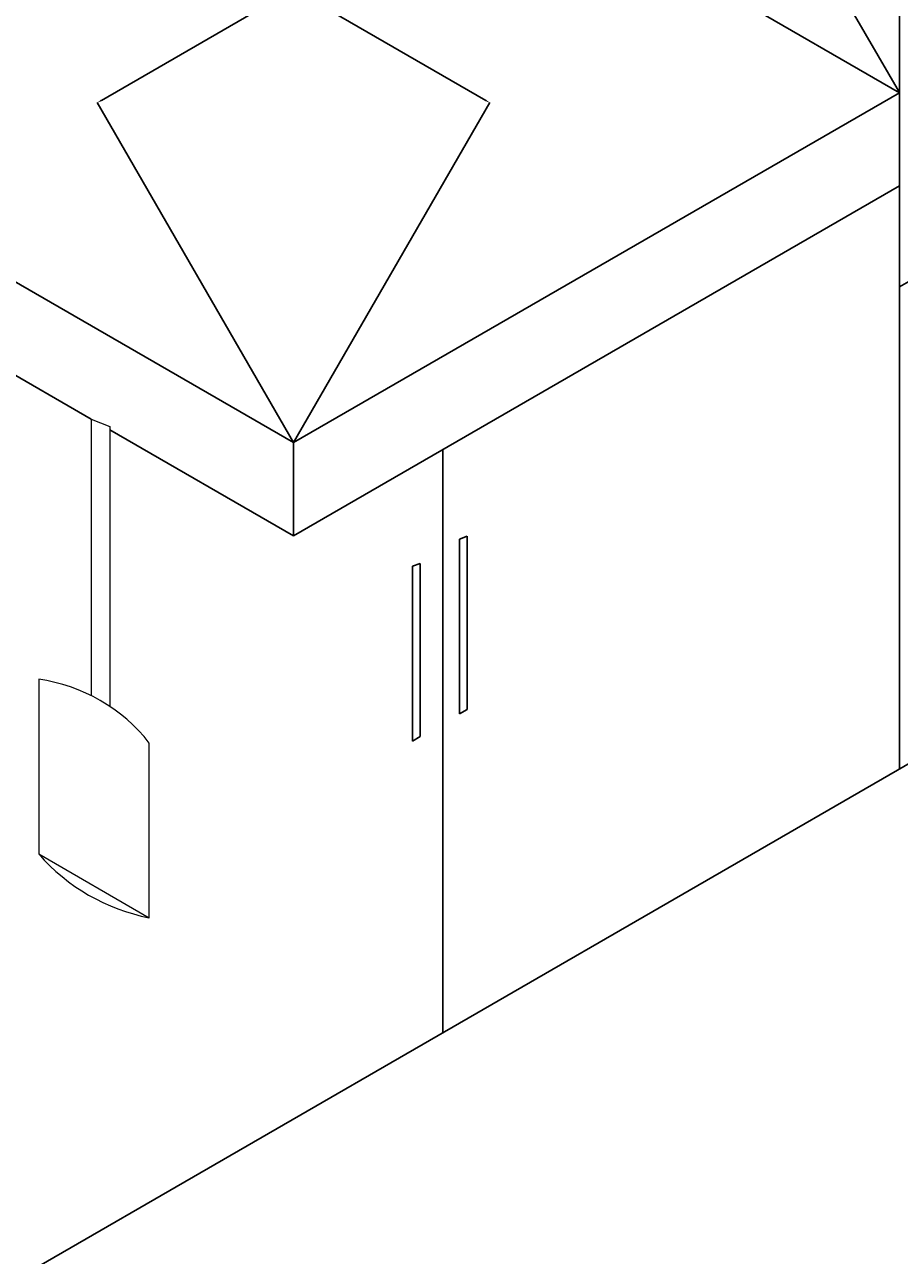
# Model space of a CAD drawing. Units: metres. Extents: x -2391 to 4922, y -635 to 4845.
# Tile 17 of 37: x -719 to 31, y 1408 to 2464. Entities that reach past the tile are written whole.
import ezdxf

# ---------------------------------------------------------------- set-up
doc = ezdxf.new("R2010")
doc.units = ezdxf.units.M
doc.header["$MEASUREMENT"] = 0
for name, color, linetype, lineweight in [('A-ANNO-DIMS', 2, 'Continuous', 18), ('A-EQPM', 9, 'Continuous', 18), ('A-FLOR-FIXT', 3, 'Continuous', 25)]:
    doc.layers.add(name, color=color, linetype=linetype, lineweight=lineweight)
doc.styles.get("Standard").update_dxf_attribs({"font": 'arial.ttf'})
doc.dimstyles.get("Standard").update_dxf_attribs({"dimtxt": 5, "dimasz": 4, "dimexe": 0.18, "dimexo": 0.0625, "dimgap": 0.09, "dimtad": 0, "dimtih": 1, "dimtoh": 1, "dimdec": 0, "dimzin": 0, "dimdsep": 46, "dimtxsty": 'Standard', "dimcen": 0.09, "dimadec": 0, "dimazin": 0, "dimtfac": 1, "dimtdec": 0, "dimtofl": 0, "dimtmove": 0, "dimatfit": 3, "dimfxl": 1, "dimtolj": 1, "dimtzin": 0, "dimarcsym": 0})

# ---------------------------------------------------------------- blocks, each defined once
blk = doc.blocks.new('UTENSIL-HANGING')
for p, q in [((0, 204.5), (0, 54.7)), ((94.7, 0), (94.7, 149.8)), ((0, 54.7), (94.7, 0))]:
    blk.add_line(p, q)
for centre, radius, start, end in [((-21.4, 58), 148.1, 38.3202, 81.6798), ((126.8, 165), 168.1, 221.0072, 258.9928)]:
    blk.add_arc(centre, radius, start, end)
blk = doc.blocks.new('HANDLE-DRAWER-152')
for p, q in [((6.8, 152.4), (0, 150)), ((0, 150), (0, 0)), ((6.8, 3.9), (6.8, 152.4)), ((0, 0), (6.8, 3.9))]:
    blk.add_line(p, q)
blk = doc.blocks.new('*D8')
at = {"layer": 'A-ANNO-DIMS', "color": 0, "lineweight": -2, "transparency": 16777216}
for p, q in [((-2047.3, 3005.2), (-2047.3, -631.4)), ((4577.8, 2350.2), (4577.8, -631.4)), ((-2043.3, -631.2), (1257.6, -631.2)), ((4573.8, -631.2), (1272.8, -631.2))]:
    blk.add_line(p, q, dxfattribs=at)
at = {"layer": 'A-ANNO-DIMS', "color": 0, "transparency": 16777216}
for points in [[(-2043.3, -630.6), (-2043.3, -631.9), (-2047.3, -631.2)], [(4573.8, -630.6), (4573.8, -631.9), (4577.8, -631.2)]]:
    blk.add_solid(points, dxfattribs=at)
at = {"layer": 'Defpoints', "color": 0, "transparency": 16777216}
for p in [(-2047.3, 3005.3), (4577.8, 2350.3), (4577.8, -631.2)]:
    blk.add_point(p, dxfattribs=at)
at = {"layer": 'A-ANNO-DIMS', "color": 0, "transparency": 16777216, "insert": (1265.2, -631.2), "char_height": 5, "attachment_point": 5}
blk.add_mtext('\\A1;6625', dxfattribs=at)
blk = doc.blocks.new('*D10')
at = {"layer": 'A-ANNO-DIMS', "color": 0, "lineweight": -2, "transparency": 16777216}
for p, q in [((550.7, 4505.3), (-2384, 4505.3)), ((-2383.8, 4501.3), (-2383.8, 2107.9)), ((-2383.8, -290.7), (-2383.8, 2102.6)), ((-488.6, -294.7), (-2384, -294.7))]:
    blk.add_line(p, q, dxfattribs=at)
at = {"layer": 'A-ANNO-DIMS', "color": 0, "transparency": 16777216}
for points in [[(-2384.5, 4501.3), (-2383.2, 4501.3), (-2383.8, 4505.3)], [(-2384.5, -290.7), (-2383.2, -290.7), (-2383.8, -294.7)]]:
    blk.add_solid(points, dxfattribs=at)
at = {"layer": 'Defpoints', "color": 0, "transparency": 16777216}
for p in [(-2383.8, 4505.3), (550.7, 4505.3), (-488.5, -294.7)]:
    blk.add_point(p, dxfattribs=at)
at = {"layer": 'A-ANNO-DIMS', "color": 0, "transparency": 16777216, "insert": (-2383.8, 2105.3), "char_height": 5, "attachment_point": 5}
blk.add_mtext('\\A1;4800', dxfattribs=at)
blk = doc.blocks.new('*D41')
at = {"layer": 'A-ANNO-DIMS', "color": 0, "lineweight": -2, "transparency": 16777216}
for p, q in [((-2047.3, 3005.3), (-1879, 3296.8)), ((-1875.6, 3294.7), (-1104.2, 2849.3)), ((-323.7, 2398.7), (-1095.1, 2844.1)), ((-488.5, 2105.3), (-320.1, 2396.8))]:
    blk.add_line(p, q, dxfattribs=at)
at = {"layer": 'A-ANNO-DIMS', "color": 0, "transparency": 16777216}
for points in [[(-1875.3, 3295.3), (-1876, 3294.1), (-1879.1, 3296.7)], [(-323.4, 2399.3), (-324, 2398.1), (-320.2, 2396.7)]]:
    blk.add_solid(points, dxfattribs=at)
at = {"layer": 'Defpoints', "color": 0, "transparency": 16777216}
for p in [(-2047.3, 3005.3), (-320.2, 2396.7), (-488.5, 2105.3)]:
    blk.add_point(p, dxfattribs=at)
at = {"layer": 'A-ANNO-DIMS', "color": 0, "transparency": 16777216, "insert": (-1099.7, 2846.7), "char_height": 5, "attachment_point": 5}
blk.add_mtext('\\A1;1800', dxfattribs=at)
blk = doc.blocks.new('*D42')
at = {"layer": 'A-ANNO-DIMS', "color": 0, "lineweight": -2, "transparency": 16777216}
for p, q in [((-140.6, 2694.7), (-392.4, 2549.3)), ((31.1, 2405.3), (-137.2, 2696.8)), ((-653.3, 2398.7), (-401.5, 2544.1)), ((-488.5, 2105.3), (-656.8, 2396.8))]:
    blk.add_line(p, q, dxfattribs=at)
at = {"layer": 'A-ANNO-DIMS', "color": 0, "transparency": 16777216}
for points in [[(-140.9, 2695.3), (-140.3, 2694.1), (-137.1, 2696.7)], [(-653.6, 2399.3), (-652.9, 2398.1), (-656.7, 2396.7)]]:
    blk.add_solid(points, dxfattribs=at)
at = {"layer": 'Defpoints', "color": 0, "transparency": 16777216}
for p in [(-137.1, 2696.7), (31.1, 2405.3), (-488.5, 2105.3)]:
    blk.add_point(p, dxfattribs=at)
at = {"layer": 'A-ANNO-DIMS', "color": 0, "transparency": 16777216, "insert": (-396.9, 2546.7), "char_height": 5, "attachment_point": 5}
blk.add_mtext('\\A1;600', dxfattribs=at)
blk = doc.blocks.new('*D46')
at = {"layer": 'A-ANNO-DIMS', "color": 0, "lineweight": -2, "transparency": 16777216}
for p, q in [((-2047.3, 1505.3), (-1887.1, 1801.4)), ((-1883.7, 1799.3), (-1087.4, 1368.5)), ((-281.2, 932.4), (-1077.6, 1363.2)), ((-437.8, 634.6), (-277.6, 930.6))]:
    blk.add_line(p, q, dxfattribs=at)
at = {"layer": 'A-ANNO-DIMS', "color": 0, "transparency": 16777216}
for points in [[(-1883.4, 1799.9), (-1884, 1798.7), (-1887.2, 1801.2)], [(-280.9, 933), (-281.6, 931.8), (-277.7, 930.5)]]:
    blk.add_solid(points, dxfattribs=at)
at = {"layer": 'Defpoints', "color": 0, "transparency": 16777216}
for p in [(-2047.3, 1505.3), (-277.7, 930.5), (-437.8, 634.5)]:
    blk.add_point(p, dxfattribs=at)
at = {"layer": 'A-ANNO-DIMS', "color": 0, "transparency": 16777216, "insert": (-1082.5, 1365.9), "char_height": 5, "attachment_point": 5}
blk.add_mtext('\\A1;1830', dxfattribs=at)

msp = doc.modelspace()

# ---------------------------------------------------------------- linework, layer by layer
at = {"layer": 'A-EQPM'}
for p, q in [((-661.9459, 2125.4219), (-646.0506, 2119.0402)), ((-661.9459, 2125.4219), (-661.9459, 1888.1658)), ((-646.0506, 2119.0402), (-646.0506, 1878.9078))]:
    msp.add_line(p, q, dxfattribs=at)
at = {"layer": 'A-FLOR-FIXT'}
for p, q in [((-1527.7191, 3305.2763), (31.1266, 2405.2763)), ((-2047.3343, 3005.2763), (-488.4886, 2105.2763)), ((31.1266, 1825.2763), (31.1266, 2652.3633)), ((31.1266, 2238.8198), (550.7419, 2536.5981)), ((-488.4886, 2105.2763), (31.1266, 2405.2763)), ((31.1266, 2405.2763), (31.1266, 2325.2763)), ((-488.4886, 2025.2763), (31.1266, 2325.2763)), ((-661.9459, 2125.4219), (-952.2504, 2293.0293)), ((550.7419, 2125.2763), (-765.6167, 1365.2763)), ((-488.4886, 2025.2763), (-646.0506, 2116.2447)), ((-488.4886, 2105.2763), (-488.4886, 2025.2763)), ((-360.3754, 2099.2424), (-360.3754, 1599.2424))]:
    msp.add_line(p, q, dxfattribs=at)

# ---------------------------------------------------------------- block references
at = {"layer": 'A-EQPM'}
msp.add_blockref('UTENSIL-HANGING', (-706.9508, 1697.8086), dxfattribs=at)
at = {"layer": 'A-FLOR-FIXT'}
for p in [(-346.283, 1872.557), (-386.5724, 1849.2959)]:
    msp.add_blockref('HANDLE-DRAWER-152', p, dxfattribs=at)

# ---------------------------------------------------------------- dimensions: what is measured, and where the dimension line sits
at = {"layer": 'A-ANNO-DIMS'}
for base, p1, p2, angle, picture, middle in [((-2383.8343, 4505.2763), (-488.4886, -294.7237), (550.7419, 4505.2763), 90, '*D10', (-2383.8343, 2105.2763)), ((-320.2386, 2396.6938), (-2047.3343, 3005.2763), (-488.4886, 2105.2763), 330, '*D41', (-1099.6615, 2846.6938)), ((-137.1234, 2696.6938), (-488.4886, 2105.2763), (31.1266, 2405.2763), 30, '*D42', (-396.931, 2546.6938)), ((-277.7211, 930.4802), (-2047.3343, 1505.2763), (-437.841, 634.5176), 331.5859855, '*D46', (-1082.4677, 1365.8595))]:
    dim = msp.add_linear_dim(base=base, p1=p1, p2=p2, angle=angle, dimstyle='Standard', override={"dimdec": 0, "dimlfac": 1, "dimrnd": 0, "dimzin": 0, "dimdsep": 46, "dimlunit": 2}, dxfattribs=at)
    dim.commit()
    dim.dimension.update_dxf_attribs({"geometry": picture, "text_midpoint": middle})
dim = msp.add_linear_dim(base=(4577.76, -631.2237), p1=(-2047.3343, 3005.2763), p2=(4577.76, 2350.2763), dimstyle='Standard', override={"dimdec": 0, "dimlfac": 1, "dimrnd": 0, "dimzin": 0, "dimdsep": 46, "dimlunit": 2}, dxfattribs=at)
dim.commit()
dim.dimension.update_dxf_attribs({"geometry": '*D8', "text_midpoint": (1265.2128, -631.2237)})

doc.saveas('drawing.dxf')
